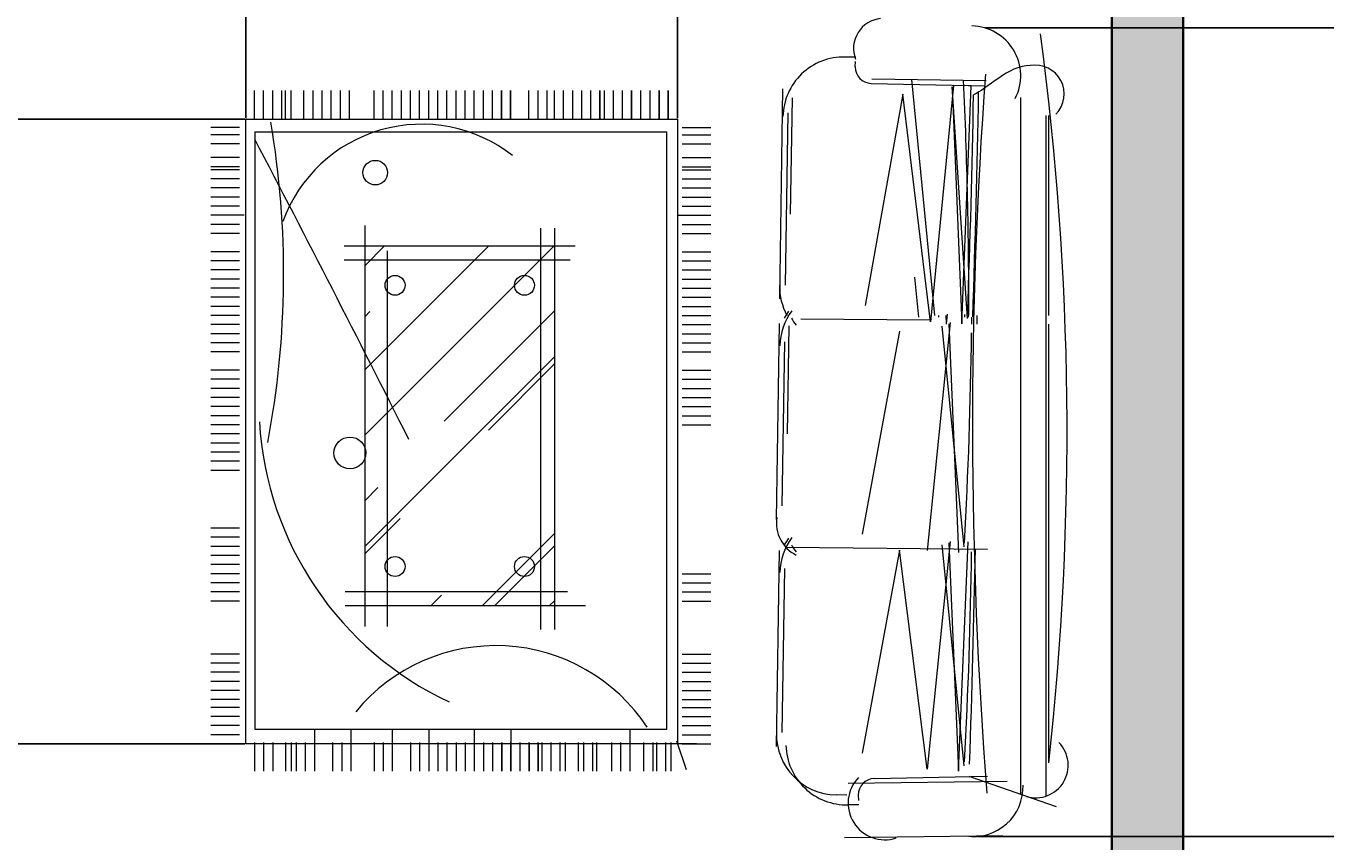
# Model space of a CAD drawing. Units: inches. Extents: x 2807 to 3326, y 2005 to 2580.
# Tile 5 of 12: x 3067 to 3149, y 2192 to 2243. Entities that reach past the tile are written whole.
import ezdxf

# ---------------------------------------------------------------- set-up
doc = ezdxf.new("R2010")
doc.units = ezdxf.units.IN
doc.header["$LTSCALE"] = 0.4
for name, color, linetype, lineweight in [('A-ANNO-DIMS', 2, 'Continuous', 18), ('A-FURN-PATT', 7, 'Continuous', 15), ('A-WALL-PATT', 231, 'Continuous', 13), ('Furniture', 7, 'Continuous', 15), ('WALL', 233, 'Continuous', 35)]:
    doc.layers.add(name, color=color, linetype=linetype, lineweight=lineweight)
doc.styles.get("Standard").update_dxf_attribs({"font": 'txt', "height": 5})
doc.dimstyles.get("Standard").update_dxf_attribs({"dimtxt": 0.18, "dimasz": 0.18, "dimexe": 0.18, "dimexo": 0.0625, "dimgap": 0.09, "dimtad": 0, "dimtih": 1, "dimtoh": 1, "dimdec": 4, "dimzin": 0, "dimdsep": 46, "dimtxsty": 'Standard', "dimcen": 0.09, "dimadec": 0, "dimazin": 0, "dimtfac": 1, "dimtdec": 4, "dimtofl": 0, "dimtmove": 0, "dimatfit": 3, "dimfxl": 1, "dimtolj": 1, "dimtzin": 0, "dimarcsym": 0})

# ---------------------------------------------------------------- blocks, each defined once
blk = doc.blocks.new('*D61')
at = {"layer": 'A-ANNO-DIMS', "color": 0, "lineweight": -2, "ltscale": 0.4, "transparency": 16777216}
for p, q in [((3088.922898, 2267.452063), (2816.937191, 2267.452063)), ((2817.117191, 2267.272063), (2817.117191, 2223.175564)), ((2817.117191, 2173.899065), (2817.117191, 2217.995564)), ((3079.479513, 2173.719065), (2816.937191, 2173.719065))]:
    blk.add_line(p, q, dxfattribs=at)
at = {"layer": 'A-ANNO-DIMS', "color": 0, "ltscale": 0.4, "transparency": 16777216}
for points in [[(2817.087191, 2267.272063), (2817.147191, 2267.272063), (2817.117191, 2267.452063)], [(2817.087191, 2173.899065), (2817.147191, 2173.899065), (2817.117191, 2173.719065)]]:
    blk.add_solid(points, dxfattribs=at)
at = {"layer": 'Defpoints', "color": 0, "ltscale": 0.4, "transparency": 16777216}
for p in [(2817.117191, 2267.452063), (3088.985398, 2267.452063), (3079.542013, 2173.719065)]:
    blk.add_point(p, dxfattribs=at)
at = {"layer": 'A-ANNO-DIMS', "color": 0, "ltscale": 0.4, "transparency": 16777216, "insert": (2817.117191, 2220.585564), "char_height": 5, "attachment_point": 5}
blk.add_mtext('\\A1;93.73', dxfattribs=at)
blk = doc.blocks.new('*D63')
at = {"layer": 'A-ANNO-DIMS', "color": 0, "lineweight": -2, "ltscale": 0.4, "transparency": 16777216}
for p, q in [((3127.088436, 2243.315958), (3316.197191, 2243.315958)), ((3316.017191, 2243.135958), (3316.017191, 2220.404674)), ((3316.017191, 2192.49339), (3316.017191, 2215.224674)), ((3126.620717, 2192.31339), (3316.197191, 2192.31339))]:
    blk.add_line(p, q, dxfattribs=at)
at = {"layer": 'A-ANNO-DIMS', "color": 0, "ltscale": 0.4, "transparency": 16777216}
for points in [[(3315.987191, 2243.135958), (3316.047191, 2243.135958), (3316.017191, 2243.315958)], [(3315.987191, 2192.49339), (3316.047191, 2192.49339), (3316.017191, 2192.31339)]]:
    blk.add_solid(points, dxfattribs=at)
at = {"layer": 'Defpoints', "color": 0, "ltscale": 0.4, "transparency": 16777216}
for p in [(3127.025936, 2243.315958), (3316.017191, 2243.315958), (3126.558217, 2192.31339)]:
    blk.add_point(p, dxfattribs=at)
at = {"layer": 'A-ANNO-DIMS', "color": 0, "ltscale": 0.4, "transparency": 16777216, "insert": (3316.017191, 2217.814674), "char_height": 5, "attachment_point": 5}
blk.add_mtext('\\A1;51', dxfattribs=at)
blk = doc.blocks.new('*D64')
at = {"layer": 'A-ANNO-DIMS', "color": 0, "lineweight": -2, "ltscale": 0.4, "transparency": 16777216}
for p, q in [((3080.426, 2237.614), (3080.426, 2577.206)), ((3080.606, 2577.026), (3081.577, 2577.026)), ((3107.489, 2577.026), (3106.519, 2577.026)), ((3107.669, 2237.614), (3107.669, 2577.206))]:
    blk.add_line(p, q, dxfattribs=at)
at = {"layer": 'A-ANNO-DIMS', "color": 0, "ltscale": 0.4, "transparency": 16777216}
for points in [[(3080.606, 2577.056), (3080.606, 2576.996), (3080.426, 2577.026)], [(3107.489, 2577.056), (3107.489, 2576.996), (3107.669, 2577.026)]]:
    blk.add_solid(points, dxfattribs=at)
at = {"layer": 'Defpoints', "color": 0, "ltscale": 0.4, "transparency": 16777216}
for p in [(3107.669, 2577.026), (3080.426, 2237.552), (3107.669, 2237.552)]:
    blk.add_point(p, dxfattribs=at)
at = {"layer": 'A-ANNO-DIMS', "color": 0, "ltscale": 0.4, "transparency": 16777216, "insert": (3094.048, 2577.026), "char_height": 5, "attachment_point": 5}
blk.add_mtext('\\A1;27.243', dxfattribs=at)
blk = doc.blocks.new('*D65')
at = {"layer": 'A-ANNO-DIMS', "color": 0, "lineweight": -2, "ltscale": 0.4, "transparency": 16777216}
for p, q in [((3080.364, 2237.552), (2816.937, 2237.552)), ((2817.117, 2237.372), (2817.117, 2220.442)), ((2817.117, 2198.333), (2817.117, 2215.262)), ((3080.364, 2198.153), (2816.937, 2198.153))]:
    blk.add_line(p, q, dxfattribs=at)
at = {"layer": 'A-ANNO-DIMS', "color": 0, "ltscale": 0.4, "transparency": 16777216}
for points in [[(2817.087, 2237.372), (2817.147, 2237.372), (2817.117, 2237.552)], [(2817.087, 2198.333), (2817.147, 2198.333), (2817.117, 2198.153)]]:
    blk.add_solid(points, dxfattribs=at)
at = {"layer": 'Defpoints', "color": 0, "ltscale": 0.4, "transparency": 16777216}
for p in [(2817.117, 2237.552), (3080.426, 2237.552), (3080.426, 2198.153)]:
    blk.add_point(p, dxfattribs=at)
at = {"layer": 'A-ANNO-DIMS', "color": 0, "ltscale": 0.4, "transparency": 16777216, "insert": (2817.117, 2217.852), "char_height": 5, "attachment_point": 5}
blk.add_mtext('\\A1;39.4', dxfattribs=at)

msp = doc.modelspace()

# ---------------------------------------------------------------- hatches: boundary and pattern name
at = {"layer": 'A-FURN-PATT'}
h = msp.add_hatch(dxfattribs=at)
h.set_pattern_fill('AR-RROOF', color=256, scale=0.310303, angle=585, style=0)
h.set_pattern_definition([(225, (4533.939, 2597.69), (-6.687848, -17.83426), [118.22556, -15.7634, 39.4085, -7.8817]), (225, (4529.314, 2587.491), (12.98557, -1.83916), [23.6451, -2.60096, 47.29022, -5.91128]), (225, (4535.89, 2590.1666), (-25.246625, -32.714721), [63.05363, -11.03439, 31.52682, -7.8817])])
h.paths.add_polyline_path([(3087.9516, 2206.8517), (3099.9018, 2206.8517), (3099.9018, 2229.5605), (3087.9516, 2229.5605)])
at = {"layer": 'A-WALL-PATT', "ltscale": 0.4}
h = msp.add_hatch(color=256, dxfattribs=at)
h.dxf.hatch_style = 1
h.paths.add_polyline_path([(3288.5672, 2549.5765), (2941.5672, 2549.5765), (2941.5672, 2540.5765), (2993.5672, 2540.5765), (2993.5672, 2489.5693), (2998.0672, 2489.5693), (2998.0672, 2540.5765), (3135.0672, 2540.5765), (3135.0672, 2479.0765), (3139.5672, 2479.0765), (3139.5672, 2540.5765), (3279.5672, 2540.5765), (3279.5672, 2510.5765), (3288.5672, 2510.5765)])
h.paths.add_polyline_path([(2905.5672, 2549.5765), (2844.5672, 2549.5765), (2844.5672, 2445.94), (2853.5672, 2445.94), (2853.5672, 2540.5765), (2905.5672, 2540.5765)])
h.paths.add_polyline_path([(2853.5672, 2409.94), (2844.5672, 2409.94), (2844.5672, 2371.3497), (2853.5672, 2371.3497), (2853.5672, 2380.0765), (2909.0672, 2380.0765), (2909.0672, 2384.5765), (2853.5672, 2384.5765)])
h.paths.add_polyline_path([(2998.0672, 2389.0765), (2993.5672, 2389.0765), (2993.5672, 2384.5765), (2939.0672, 2384.5765), (2939.0672, 2380.0765), (2943.5672, 2380.0765), (2943.5672, 2314.0765), (2948.0672, 2314.0765), (2948.0672, 2380.0765), (2998.0672, 2380.0765)])
h.paths.add_polyline_path([(2998.0672, 2471.8029), (2993.5672, 2471.8029), (2993.5672, 2425.0765), (2998.0672, 2425.0765)])
h.paths.add_polyline_path([(2953.0672, 2279.5765), (2948.0672, 2279.5765), (2948.0672, 2284.0765), (2943.5672, 2284.0765), (2943.5672, 2279.5765), (2853.5672, 2279.5765), (2853.5672, 2289.0663), (2844.5672, 2289.0663), (2844.5672, 2227.8961), (2853.5672, 2227.8961), (2853.5672, 2275.0765), (2953.0672, 2275.0765)])
h.paths.add_polyline_path([(2943.5672, 2332.0765), (2853.5672, 2332.0765), (2853.5672, 2347.3497), (2844.5672, 2347.3497), (2844.5672, 2313.0663), (2853.5672, 2313.0663), (2853.5672, 2327.5765), (2943.5672, 2327.5765)])
h.paths.add_polyline_path([(3144.0672, 2279.5765), (2993.5672, 2279.5765), (2989.0672, 2279.5765), (2989.0672, 2275.0765), (2993.5672, 2275.0765), (2993.5672, 2144.5765), (2984.5672, 2144.5765), (2984.5672, 2135.5765), (2993.5672, 2135.5765), (2993.5672, 2120.0765), (3036.5672, 2120.0765), (3036.5672, 2129.0765), (2998.0672, 2129.0765), (2998.0672, 2275.0765), (3135.0672, 2275.0765), (3135.0672, 2129.0765), (3096.5672, 2129.0765), (3096.5672, 2120.0765), (3139.5672, 2120.0765), (3139.5672, 2135.5765), (3148.5672, 2135.5765), (3148.5672, 2144.5765), (3139.5672, 2144.5765), (3139.5672, 2275.0765), (3144.0672, 2275.0765)])
h.paths.add_polyline_path([(2984.5672, 2144.5765), (2925.9914, 2144.5765), (2925.9914, 2135.5765), (2984.5672, 2135.5765)])
h.paths.add_polyline_path([(2889.9914, 2144.5765), (2853.5672, 2144.5765), (2853.5672, 2191.8961), (2844.5672, 2191.8961), (2844.5672, 2135.5765), (2889.9914, 2135.5765)])
h.paths.add_polyline_path([(3196.0672, 2144.5765), (3148.5672, 2144.5765), (3148.5672, 2135.5765), (3196.0672, 2135.5765)])
h.paths.add_polyline_path([(3288.5672, 2191.8265), (3279.5672, 2191.8265), (3279.5672, 2144.5765), (3232.0672, 2144.5765), (3232.0672, 2135.5765), (3288.5672, 2135.5765)])
h.paths.add_polyline_path([(3288.5672, 2292.8229), (3279.5672, 2292.8229), (3279.5672, 2291.4371), (3279.5672, 2279.5765), (3189.5672, 2279.5765), (3189.5672, 2293.0765), (3185.0672, 2293.0765), (3185.0672, 2279.5765), (3180.0672, 2279.5765), (3180.0672, 2275.0765), (3279.5672, 2275.0765), (3279.5672, 2227.8265), (3288.5672, 2227.8265)])
h.paths.add_polyline_path([(3288.5672, 2368.0765), (3279.5672, 2368.0765), (3279.5672, 2332.0765), (3174.0672, 2332.0765), (3174.0672, 2327.5765), (3185.0672, 2327.5765), (3189.5672, 2327.5765), (3279.5672, 2327.5765), (3279.5672, 2316.8229), (3288.5672, 2316.8229)])
h.paths.add_polyline_path([(3288.5672, 2474.5765), (3279.5672, 2474.5765), (3279.5672, 2444.5765), (3139.5672, 2444.5765), (3139.5672, 2449.0765), (3135.0672, 2449.0765), (3135.0672, 2327.5765), (3144.0672, 2327.5765), (3144.0672, 2332.0765), (3139.5672, 2332.0765), (3139.5672, 2440.0765), (3279.5672, 2440.0765), (3279.5672, 2404.0765), (3288.5672, 2404.0765)])

# ---------------------------------------------------------------- linework, layer by layer
at = {"layer": 'Furniture'}
for p, q in [((3118.9148, 2241.4623), (3118.2308, 2241.4765)), ((3118.8729, 2240.8649), (3118.8798, 2241.1972)), ((3114.2777, 2239.4771), (3114.0864, 2226.2182)), ((3119.8798, 2239.8154), (3127.0319, 2239.6674)), ((3119.9106, 2240.1104), (3127.142, 2239.9866)), ((3123.8848, 2225.1761), (3122.4439, 2240.067)), ((3125.07, 2239.6772), (3123.6184, 2224.7734)), ((3125.9472, 2224.9922), (3124.9824, 2239.5925)), ((3124.9824, 2239.5925), (3125.5969, 2224.6533)), ((3126.1891, 2239.658), (3125.07, 2239.6772)), ((3125.5969, 2224.6533), (3126.1891, 2239.658)), ((3080.9833, 2237.5598), (3080.9833, 2239.3694)), ((3081.5581, 2237.5598), (3081.5581, 2239.3694)), ((3082.133, 2237.5598), (3082.133, 2239.3694)), ((3082.7078, 2237.5598), (3082.7078, 2239.3694)), ((3082.927, 2237.5598), (3082.927, 2239.3694)), ((3083.2827, 2237.5598), (3083.2827, 2239.3694)), ((3084.0989, 2237.5598), (3084.0989, 2239.3694)), ((3084.6737, 2237.5598), (3084.6737, 2239.3694)), ((3085.2486, 2237.5598), (3085.2486, 2239.3694)), ((3085.8234, 2237.5598), (3085.8234, 2239.3694)), ((3086.3982, 2237.5598), (3086.3982, 2239.3694)), ((3086.9731, 2237.5598), (3086.9731, 2239.3694)), ((3088.5232, 2237.5598), (3088.5232, 2239.3694)), ((3089.098, 2237.5598), (3089.098, 2239.3694)), ((3089.6729, 2237.5598), (3089.6729, 2239.3694)), ((3090.2477, 2237.5598), (3090.2477, 2239.3694)), ((3090.8225, 2237.5598), (3090.8225, 2239.3694)), ((3091.3974, 2237.5598), (3091.3974, 2239.3694)), ((3091.9722, 2237.5598), (3091.9722, 2239.3694)), ((3092.5471, 2237.5598), (3092.5471, 2239.3694)), ((3093.1219, 2237.5598), (3093.1219, 2239.3694)), ((3093.6967, 2237.5598), (3093.6967, 2239.3694)), ((3094.2716, 2237.5598), (3094.2716, 2239.3694)), ((3094.8464, 2237.5598), (3094.8464, 2239.3694)), ((3095.4212, 2237.5598), (3095.4212, 2239.3694)), ((3095.9961, 2237.5598), (3095.9961, 2239.3694)), ((3096.5587, 2237.5598), (3096.5587, 2239.3694)), ((3096.5709, 2237.5598), (3096.5709, 2239.3694)), ((3097.1336, 2237.5598), (3097.1336, 2239.3694)), ((3097.1458, 2237.5598), (3097.1458, 2239.3694)), ((3098.2937, 2237.5598), (3098.2937, 2239.3694)), ((3098.8685, 2237.5598), (3098.8685, 2239.3694)), ((3099.4434, 2237.5598), (3099.4434, 2239.3694)), ((3099.9025, 2237.5598), (3099.9025, 2239.3694)), ((3100.4774, 2237.5598), (3100.4774, 2239.3694)), ((3101.0522, 2237.5598), (3101.0522, 2239.3694)), ((3101.627, 2237.5598), (3101.627, 2239.3694)), ((3102.1897, 2237.5598), (3102.1897, 2239.3694)), ((3102.2019, 2237.5598), (3102.2019, 2239.3694)), ((3102.7645, 2237.5598), (3102.7645, 2239.3694)), ((3102.7767, 2237.5598), (3102.7767, 2239.3694)), ((3103.0515, 2237.5598), (3103.0515, 2239.3694)), ((3103.6263, 2237.5598), (3103.6263, 2239.3694)), ((3104.2012, 2237.5598), (3104.2012, 2239.3694)), ((3104.7638, 2237.5598), (3104.7638, 2239.3694)), ((3104.776, 2237.5598), (3104.776, 2239.3694)), ((3105.3387, 2237.5598), (3105.3387, 2239.3694)), ((3105.3508, 2237.5598), (3105.3508, 2239.3694)), ((3105.9461, 2237.5598), (3105.9461, 2239.3694)), ((3106.5087, 2237.5598), (3106.5087, 2239.3694)), ((3106.5209, 2237.5598), (3106.5209, 2239.3694)), ((3107.0836, 2237.5598), (3107.0836, 2239.3694)), ((3107.0957, 2237.5598), (3107.0957, 2239.3694)), ((3114.8954, 2238.9029), (3114.7789, 2231.5635)), ((3121.8744, 2239.1284), (3119.5024, 2225.7922)), ((3123.6184, 2224.7734), (3121.8744, 2239.1284)), ((3129.3238, 2225.1761), (3129.3238, 2238.918)), ((3114.6209, 2237.9592), (3114.4439, 2227.0859)), ((3130.9062, 2225.1761), (3130.9062, 2237.791)), ((3131.0821, 2225.1761), (3131.0821, 2237.791)), ((3080.0266, 2237.0345), (3078.217, 2237.0345)), ((3080.4262, 2237.5518), (3107.6694, 2237.5518)), ((3080.4262, 2198.1526), (3080.4262, 2237.5518)), ((3107.6694, 2237.5518), (3107.6694, 2198.1526)), ((3107.9651, 2237.0345), (3109.7748, 2237.0345)), ((3080.0266, 2236.568), (3078.217, 2236.568)), ((3080.9955, 2236.7472), (3106.9962, 2236.7472)), ((3080.9955, 2236.7472), (3080.9955, 2199.0713)), ((3106.9962, 2199.0713), (3106.9962, 2236.7472)), ((3107.9651, 2236.568), (3109.7748, 2236.568)), ((3080.0266, 2235.9931), (3078.217, 2235.9931)), ((3107.9651, 2235.9931), (3109.7748, 2235.9931)), ((3080.0266, 2235.1317), (3078.217, 2235.1317)), ((3080.0266, 2234.5568), (3078.217, 2234.5568)), ((3107.9651, 2235.1317), (3109.7748, 2235.1317)), ((3107.9651, 2234.5568), (3109.7748, 2234.5568)), ((3080.0266, 2234.3671), (3078.217, 2234.3671)), ((3080.0266, 2233.7923), (3078.217, 2233.7923)), ((3107.9651, 2234.3671), (3109.7748, 2234.3671)), ((3107.9651, 2233.7923), (3109.7748, 2233.7923)), ((3080.0266, 2233.2174), (3078.217, 2233.2174)), ((3107.9651, 2233.2174), (3109.7748, 2233.2174)), ((3080.0266, 2232.6426), (3078.217, 2232.6426)), ((3080.0266, 2232.0677), (3078.217, 2232.0677)), ((3107.9651, 2232.6426), (3109.7748, 2232.6426)), ((3107.9651, 2232.0677), (3109.7748, 2232.0677)), ((3080.3223, 2231.4929), (3078.217, 2231.4929)), ((3107.6694, 2231.4929), (3109.7748, 2231.4929)), ((3080.0266, 2230.9181), (3078.217, 2230.9181)), ((3087.9516, 2205.5436), (3087.9516, 2230.8534)), ((3099.0203, 2230.676), (3099.0203, 2205.3662)), ((3099.9018, 2230.676), (3099.9018, 2205.3662)), ((3107.9651, 2230.9181), (3109.7748, 2230.9181)), ((3080.0266, 2230.3432), (3078.217, 2230.3432)), ((3107.9651, 2230.3432), (3109.7748, 2230.3432)), ((3080.0266, 2229.1936), (3078.217, 2229.1936)), ((3086.6283, 2229.5605), (3101.2044, 2229.5605)), ((3089.3649, 2205.5436), (3089.3649, 2229.2568)), ((3107.9651, 2229.1936), (3109.7748, 2229.1936)), ((3080.0266, 2228.6187), (3078.217, 2228.6187)), ((3080.0266, 2228.0439), (3078.217, 2228.0439)), ((3086.6283, 2228.679), (3100.8912, 2228.679)), ((3107.9651, 2228.6187), (3109.7748, 2228.6187)), ((3107.9651, 2228.0439), (3109.7748, 2228.0439)), ((3080.0266, 2227.469), (3078.217, 2227.469)), ((3107.9651, 2227.469), (3109.7748, 2227.469)), ((3122.8883, 2225.0632), (3122.6352, 2227.5852)), ((3080.0266, 2226.8942), (3078.217, 2226.8942)), ((3080.0266, 2226.3194), (3078.217, 2226.3194)), ((3107.9651, 2226.8942), (3109.7748, 2226.8942)), ((3107.9651, 2226.3194), (3109.7748, 2226.3194)), ((3080.0266, 2225.7445), (3078.217, 2225.7445)), ((3107.9651, 2225.7445), (3109.7748, 2225.7445)), ((3080.0266, 2225.1697), (3078.217, 2225.1697)), ((3107.9651, 2225.1697), (3109.7748, 2225.1697)), ((3115.4372, 2224.9639), (3123.5817, 2224.8909)), ((3124.8686, 2224.7246), (3123.417, 2210.3508)), ((3124.1531, 2225.0632), (3124.1417, 2225.1761)), ((3124.5897, 2225.1659), (3124.6132, 2224.6159)), ((3124.6773, 2225.2507), (3124.6132, 2224.6159)), ((3125.7895, 2225.0632), (3125.7964, 2225.2315)), ((3126.569, 2225.0632), (3126.569, 2225.1761)), ((3126.569, 2224.6269), (3126.569, 2225.0632)), ((3129.3238, 2225.0632), (3129.3238, 2225.1761)), ((3129.3238, 2224.6269), (3129.3238, 2225.0632)), ((3130.9062, 2225.0632), (3130.9062, 2225.1761)), ((3130.9062, 2224.6269), (3130.9062, 2225.0632)), ((3080.0266, 2224.5949), (3078.217, 2224.5949)), ((3080.0266, 2224.02), (3078.217, 2224.02)), ((3107.9651, 2224.5949), (3109.7748, 2224.5949)), ((3107.9651, 2224.02), (3109.7748, 2224.02)), ((3114.0763, 2224.6587), (3113.8851, 2212.2973)), ((3114.6941, 2224.5097), (3114.5776, 2217.7004)), ((3121.6731, 2224.1757), (3119.3011, 2211.3696)), ((3125.7458, 2210.5696), (3124.3477, 2224.5038)), ((3124.7811, 2224.6398), (3125.3956, 2210.2307)), ((3129.3238, 2194.9618), (3129.3238, 2224.6269)), ((3130.9062, 2194.8553), (3130.9062, 2224.6269)), ((3131.0821, 2197.0256), (3131.0821, 2224.6269)), ((3080.0266, 2223.4452), (3078.217, 2223.4452)), ((3107.9651, 2223.4452), (3109.7748, 2223.4452)), ((3114.4196, 2223.5082), (3114.2426, 2213.1649)), ((3080.0266, 2222.8704), (3078.217, 2222.8704)), ((3107.9651, 2222.8704), (3109.7748, 2222.8704)), ((3080.0266, 2221.7207), (3078.217, 2221.7207)), ((3107.9651, 2221.7207), (3109.7748, 2221.7207)), ((3080.0266, 2221.1458), (3078.217, 2221.1458)), ((3080.0266, 2220.571), (3078.217, 2220.571)), ((3107.9651, 2221.1458), (3109.7748, 2221.1458)), ((3107.9651, 2220.571), (3109.7748, 2220.571)), ((3080.0266, 2219.9962), (3078.217, 2219.9962)), ((3107.9651, 2219.9962), (3109.7748, 2219.9962)), ((3080.0266, 2219.4213), (3078.217, 2219.4213)), ((3107.9651, 2219.4213), (3109.7748, 2219.4213)), ((3080.0266, 2218.8465), (3078.217, 2218.8465)), ((3080.0266, 2218.2717), (3078.217, 2218.2717)), ((3107.9651, 2218.8465), (3109.7748, 2218.8465)), ((3107.9651, 2218.2717), (3109.7748, 2218.2717)), ((3080.0266, 2217.6968), (3078.217, 2217.6968)), ((3080.0266, 2217.122), (3078.217, 2217.122)), ((3080.0266, 2216.5471), (3078.217, 2216.5471)), ((3080.0266, 2215.9723), (3078.217, 2215.9723)), ((3080.0266, 2215.3975), (3078.217, 2215.3975)), ((3080.0266, 2211.7553), (3078.217, 2211.7553)), ((3080.0266, 2211.1805), (3078.217, 2211.1805)), ((3124.8686, 2210.9199), (3123.417, 2196.5461)), ((3124.7811, 2210.8351), (3125.3956, 2196.426)), ((3125.3956, 2196.426), (3125.9878, 2210.9007)), ((3080.0266, 2210.6056), (3078.217, 2210.6056)), ((3080.0266, 2210.0308), (3078.217, 2210.0308)), ((3114.0763, 2210.3523), (3113.8851, 2197.9909)), ((3114.4951, 2210.5544), (3127.2232, 2210.4358)), ((3121.6731, 2210.371), (3119.3011, 2197.565)), ((3123.417, 2196.5461), (3121.6731, 2210.371)), ((3125.7458, 2196.7649), (3124.3477, 2210.6991)), ((3080.0266, 2209.4559), (3078.217, 2209.4559)), ((3114.4196, 2209.2019), (3114.2426, 2198.8586)), ((3080.0266, 2208.8811), (3078.217, 2208.8811)), ((3080.0266, 2208.3063), (3078.217, 2208.3063)), ((3107.9651, 2208.8811), (3109.7748, 2208.8811)), ((3107.9651, 2208.3063), (3109.7748, 2208.3063)), ((3080.0266, 2207.7314), (3078.217, 2207.7314)), ((3100.7139, 2207.7332), (3086.709, 2207.7332)), ((3107.9651, 2207.7314), (3109.7748, 2207.7314)), ((3080.0266, 2207.1566), (3078.217, 2207.1566)), ((3101.8622, 2206.8517), (3086.709, 2206.8517)), ((3107.9651, 2207.1566), (3109.7748, 2207.1566)), ((3080.0266, 2203.8126), (3078.217, 2203.8126)), ((3107.9651, 2203.8126), (3109.7748, 2203.8126)), ((3080.0266, 2203.2378), (3078.217, 2203.2378)), ((3080.0266, 2202.663), (3078.217, 2202.663)), ((3107.9651, 2203.2378), (3109.7748, 2203.2378)), ((3107.9651, 2202.663), (3109.7748, 2202.663)), ((3080.0266, 2202.0881), (3078.217, 2202.0881)), ((3107.9651, 2202.0881), (3109.7748, 2202.0881)), ((3080.0266, 2201.5133), (3078.217, 2201.5133)), ((3080.0266, 2200.9384), (3078.217, 2200.9384)), ((3107.9651, 2201.5133), (3109.7748, 2201.5133)), ((3107.9651, 2200.9384), (3109.7748, 2200.9384)), ((3080.0266, 2200.4487), (3078.217, 2200.4487)), ((3107.9651, 2200.4487), (3109.7748, 2200.4487)), ((3080.0266, 2199.8739), (3078.217, 2199.8739)), ((3080.0266, 2199.2991), (3078.217, 2199.2991)), ((3107.9651, 2199.8739), (3109.7748, 2199.8739)), ((3107.9651, 2199.2991), (3109.7748, 2199.2991)), ((3080.0266, 2198.7242), (3078.217, 2198.7242)), ((3080.9955, 2199.0713), (3106.9962, 2199.0713)), ((3084.7565, 2199.0713), (3084.7565, 2196.4332)), ((3087.0559, 2199.0713), (3087.0559, 2196.4332)), ((3089.6729, 2199.0713), (3089.6729, 2196.4332)), ((3091.9722, 2199.0713), (3091.9722, 2196.4332)), ((3094.8464, 2199.0713), (3094.8464, 2196.4332)), ((3097.1458, 2199.0713), (3097.1458, 2196.4332)), ((3104.6469, 2199.0713), (3104.6469, 2196.4332)), ((3107.9651, 2198.7242), (3109.7748, 2198.7242)), ((3080.0266, 2198.1494), (3078.217, 2198.1494)), ((3108.8699, 2198.1494), (3080.4262, 2198.1526)), ((3080.9833, 2198.2428), (3080.9833, 2196.4332)), ((3081.5581, 2198.2428), (3081.5581, 2196.4332)), ((3082.133, 2198.2428), (3082.133, 2196.4332)), ((3082.927, 2198.2428), (3082.927, 2196.4332)), ((3083.2827, 2198.2428), (3083.2827, 2196.4332)), ((3083.6068, 2198.2428), (3083.6068, 2196.4332)), ((3084.1817, 2198.2428), (3084.1817, 2196.4332)), ((3085.9062, 2198.2428), (3085.9062, 2196.4332)), ((3086.481, 2198.2428), (3086.481, 2196.4332)), ((3088.5232, 2198.2428), (3088.5232, 2196.4332)), ((3089.098, 2198.2428), (3089.098, 2196.4332)), ((3090.8225, 2198.2428), (3090.8225, 2196.4332)), ((3091.3974, 2198.2428), (3091.3974, 2196.4332)), ((3092.5471, 2198.2428), (3092.5471, 2196.4332)), ((3093.1219, 2198.2428), (3093.1219, 2196.4332)), ((3093.6967, 2198.2428), (3093.6967, 2196.4332)), ((3094.2716, 2198.2428), (3094.2716, 2196.4332)), ((3095.4212, 2198.2428), (3095.4212, 2196.4332)), ((3095.9961, 2198.2428), (3095.9961, 2196.4332)), ((3096.5587, 2198.2428), (3096.5587, 2196.4332)), ((3096.5709, 2198.2428), (3096.5709, 2196.4332)), ((3097.1336, 2198.2428), (3097.1336, 2196.4332)), ((3097.7084, 2198.2428), (3097.7084, 2196.4332)), ((3097.7206, 2198.2428), (3097.7206, 2196.4332)), ((3098.2833, 2198.2428), (3098.2833, 2196.4332)), ((3098.2954, 2198.2428), (3098.2954, 2196.4332)), ((3098.8581, 2198.2428), (3098.8581, 2196.4332)), ((3098.8703, 2198.2428), (3098.8703, 2196.4332)), ((3099.0942, 2198.2428), (3099.0942, 2196.4332)), ((3099.669, 2198.2428), (3099.669, 2196.4332)), ((3100.2439, 2198.2428), (3100.2439, 2196.4332)), ((3100.5826, 2198.2428), (3100.5826, 2196.4332)), ((3101.3936, 2198.2428), (3101.3936, 2196.4332)), ((3101.7323, 2198.2428), (3101.7323, 2196.4332)), ((3102.3071, 2198.2428), (3102.3071, 2196.4332)), ((3102.5432, 2198.2428), (3102.5432, 2196.4332)), ((3103.4972, 2198.2428), (3103.4972, 2196.4332)), ((3104.072, 2198.2428), (3104.072, 2196.4332)), ((3105.5211, 2198.2428), (3105.5211, 2196.4332)), ((3106.0959, 2198.2428), (3106.0959, 2196.4332)), ((3106.3321, 2198.2428), (3106.3321, 2196.4332)), ((3106.9069, 2198.2428), (3106.9069, 2196.4332)), ((3107.2456, 2198.2428), (3107.2456, 2196.4332)), ((3107.6062, 2198.3407), (3108.2134, 2196.5214)), ((3107.9651, 2198.1494), (3109.7748, 2198.1494)), ((3120.0712, 2195.9584), (3127.2232, 2196.1064)), ((3131.5686, 2194.1835), (3126.0612, 2196.0929)), ((3118.4227, 2195.6634), (3128.4557, 2195.7872)), ((3118.3452, 2194.911), (3117.6612, 2194.9251)), ((3118.3452, 2194.911), (3117.6612, 2194.9251)), ((3119.0642, 2194.9089), (3119.0711, 2194.5766)), ((3119.1062, 2194.3115), (3118.4221, 2194.2973)), ((3128.1923, 2192.3399), (3118.1852, 2192.2138))]:
    msp.add_line(p, q, dxfattribs=at)
for centre, radius in [((3088.5962, 2234.183), 0.7752), ((3089.8462, 2227.0756), 0.6291), ((3098.0072, 2227.0756), 0.6291), ((3086.9968, 2216.4987), 1.0039), ((3089.8462, 2209.3366), 0.6291), ((3098.0072, 2209.3366), 0.6291)]:
    msp.add_circle(centre, radius, dxfattribs=at)
for centre, radius, start, end in [((3120.6643, 2242.0094), 1.9033, 95.650869, 200.597543), ((3126.1704, 2240.2906), 3.1439, 332.872897, 88.814487), ((2943.9007, 2217.8342), 188.3345, 353.634969, 7.663341), ((3118.1514, 2237.6386), 3.8387, 88.814487, 178.814487), ((3119.9011, 2240.8436), 1.0285, 178.814487, 268.814487), ((3422.5006, 2218.3097), 296.2329, 175.724776, 184.505292), ((3130.2327, 2239.1429), 1.82, 315.425312, 100.014093), ((2810.7468, 2225.511), 315.2935, 359.939131, 2.635927), ((2443.8406, 2250.7541), 682.5923, 357.857629, 359.0216363), ((2095.0491, 2258.9615), 1031.7974, 358.1190452, 358.9035573), ((3026.1813, 2227.7997), 56.6376, 349.176177, 9.732781), ((3091.5186, 2227.9342), 9.3042, 51.929705, 160.044367), ((1920.6885, 1629.0919), 1309.5846, 26.692308, 27.6237536), ((3117.942, 2226.9903), 3.8387, 178.814487, 208.203806), ((3117.95, 2223.1876), 3.8387, 143.486293, 178.814487), ((3117.7587, 2223.1543), 3.8387, 143.486293, 151.168991), ((3118.1514, 2226.954), 3.8387, 210.50473, 218.408271), ((2832.8612, 2228.0597), 293.179, 359.414373, 359.436435), ((2833.0525, 2225.5323), 293.179, 359.823059, 359.908321), ((2833.0525, 2227.5336), 293.179, 356.730785, 359.322598), ((3102.1392, 2219.6879), 20.8822, 183.342071, 244.813654), ((3116.1629, 2212.0756), 2.2574, 171.240011, 243.304404), ((3117.95, 2208.8813), 3.8387, 143.486293, 178.814487), ((3117.7587, 2208.848), 3.8387, 143.486293, 151.168991), ((3118.1514, 2212.6477), 3.8387, 210.50473, 218.408271), ((2833.0525, 2213.729), 293.179, 356.730785, 359.322598), ((2170.7942, 2229.4638), 955.851, 358.0457337, 358.8608168), ((3096.1991, 2192.9069), 11.4372, 33.379039, 140.519553), ((3117.7406, 2198.763), 3.8387, 178.814487, 268.814487), ((3118.3427, 2198.1352), 3.8387, 181.185513, 271.185513), ((3130.2651, 2196.7944), 2.0424, 253.262733, 44.552919), ((3120.7416, 2194.4162), 2.3178, 136.00951, 288.153774), ((3120.0925, 2194.9302), 1.0285, 91.185513, 181.185513), ((3126.3334, 2195.4309), 3.1255, 261.465976, 2.136694)]:
    msp.add_arc(centre, radius, start, end, dxfattribs=at)
msp.add_open_spline([(3129.9162, 2240.9352), (3128.5168, 2240.9592), (3127.1895, 2239.4274), (3126.3334, 2239.0989)], degree=3, dxfattribs=at)
at = {"layer": 'WALL'}
for p, q in [((3135.0672, 2275.0765), (3135.0672, 2129.0765)), ((3139.5672, 2275.0765), (3139.5672, 2144.5765))]:
    msp.add_line(p, q, dxfattribs=at)

# ---------------------------------------------------------------- dimensions: what is measured, and where the dimension line sits
at = {"layer": 'A-ANNO-DIMS', "ltscale": 0.4}
dim = msp.add_linear_dim(base=(3107.6694, 2577.0265), p1=(3080.4262, 2237.5518), p2=(3107.6694, 2237.5518), dimstyle='Standard', override={"dimdec": 3, "dimlfac": 1, "dimrnd": 0, "dimzin": 0, "dimdsep": 46, "dimlunit": 2}, dxfattribs=at)
dim.commit()
dim.dimension.update_dxf_attribs({"geometry": '*D64', "text_midpoint": (3094.0478, 2577.0265)})
for base, p1, p2, override, picture, middle in [((2817.1172, 2267.4521), (3079.542, 2173.7191), (3088.9854, 2267.4521), {"dimdec": 2, "dimlfac": 1, "dimrnd": 0, "dimzin": 0, "dimdsep": 46, "dimlunit": 2}, '*D61', (2817.1172, 2220.5856)), ((3316.0172, 2243.316), (3126.5582, 2192.3134), (3127.0259, 2243.316), {"dimdec": 0, "dimlfac": 1, "dimrnd": 0, "dimzin": 0, "dimdsep": 46, "dimlunit": 2}, '*D63', (3316.0172, 2217.8147)), ((2817.1172, 2237.5518), (3080.4262, 2198.1526), (3080.4262, 2237.5518), {"dimdec": 1, "dimlfac": 1, "dimrnd": 0, "dimzin": 0, "dimdsep": 46, "dimlunit": 2}, '*D65', (2817.1172, 2217.8522))]:
    dim = msp.add_linear_dim(base=base, p1=p1, p2=p2, angle=90, dimstyle='Standard', override=override, dxfattribs=at)
    dim.commit()
    dim.dimension.update_dxf_attribs({"geometry": picture, "text_midpoint": middle})

doc.saveas('drawing.dxf')
